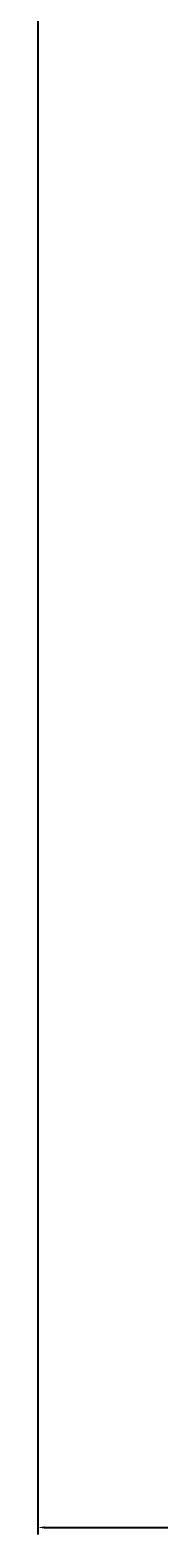
# Model space of a CAD drawing. Units: inches. Extents: x -173 to 545, y -746 to 104.
# Tile 3 of 32: x 220 to 223, y -741 to -702. Entities that reach past the tile are written whole.
import ezdxf

# ---------------------------------------------------------------- set-up
doc = ezdxf.new("R2010")
doc.units = ezdxf.units.IN
doc.header["$MEASUREMENT"] = 0
doc.layers.add('A-ANNO-DIMS', color=2, linetype='Continuous', lineweight=18)
doc.styles.get("Standard").update_dxf_attribs({"font": 'arial.ttf'})
doc.dimstyles.get("Standard").update_dxf_attribs({"dimtxt": 0.18, "dimasz": 0.18, "dimexe": 0.18, "dimexo": 0.0625, "dimgap": 0.09, "dimtad": 0, "dimtih": 1, "dimtoh": 1, "dimdec": 0, "dimzin": 0, "dimdsep": 46, "dimlunit": 3, "dimtxsty": 'Standard', "dimcen": 0.09, "dimadec": 0, "dimazin": 0, "dimtfac": 1, "dimtdec": 0, "dimtofl": 0, "dimtmove": 0, "dimatfit": 3, "dimfxl": 1, "dimtolj": 1, "dimtzin": 0, "dimarcsym": 0})

# ---------------------------------------------------------------- blocks, each defined once
blk = doc.blocks.new('*D81')
at = {"layer": 'A-ANNO-DIMS', "color": 0, "lineweight": -2, "transparency": 16777216}
for p, q in [((219.801, -551.924), (219.801, -740.642)), ((306.301, -551.924), (306.301, -740.642)), ((219.981, -740.462), (262.513, -740.462)), ((306.121, -740.462), (263.59, -740.462))]:
    blk.add_line(p, q, dxfattribs=at)
at = {"layer": 'A-ANNO-DIMS', "color": 0, "transparency": 16777216}
for points in [[(219.981, -740.432), (219.981, -740.492), (219.801, -740.462)], [(306.121, -740.432), (306.121, -740.492), (306.301, -740.462)]]:
    blk.add_solid(points, dxfattribs=at)
at = {"layer": 'Defpoints', "color": 0, "transparency": 16777216}
for p in [(219.801, -551.862), (306.301, -551.862), (306.301, -740.462)]:
    blk.add_point(p, dxfattribs=at)
at = {"layer": 'A-ANNO-DIMS', "color": 0, "transparency": 16777216, "insert": (263.051, -740.462), "char_height": 0.18, "attachment_point": 5}
blk.add_mtext('\\A1;7\'-2 1/2"', dxfattribs=at)

msp = doc.modelspace()

# ---------------------------------------------------------------- dimensions: what is measured, and where the dimension line sits
at = {"layer": 'A-ANNO-DIMS'}
dim = msp.add_linear_dim(base=(306.301, -740.462), p1=(219.801, -551.862), p2=(306.301, -551.862), dimstyle='Standard', override={"dimdec": 1, "dimlfac": 1, "dimrnd": 0, "dimzin": 1, "dimdsep": 46, "dimlunit": 4, "dimfrac": 2}, dxfattribs=at)
dim.commit()
dim.dimension.update_dxf_attribs({"geometry": '*D81', "text_midpoint": (263.051, -740.462)})

doc.saveas('drawing.dxf')
